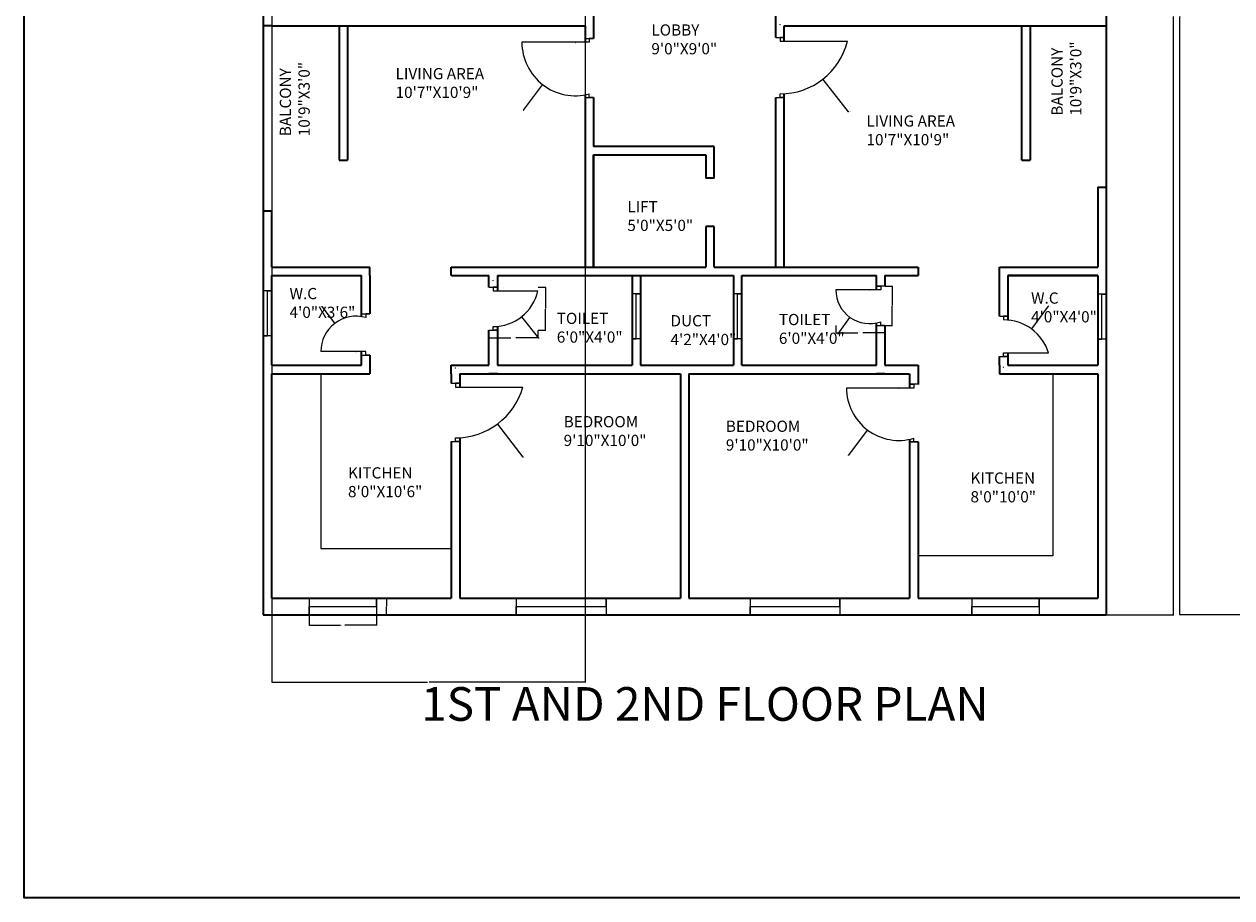
# Model space of a CAD drawing. Units: inches. Extents: x 2043 to 3387, y 1535 to 2797.
# Tile 1 of 7: x 2043 to 2688, y 1535 to 2002. Entities that reach past the tile are written whole.
import ezdxf

# ---------------------------------------------------------------- set-up
doc = ezdxf.new("R2010")
doc.units = ezdxf.units.IN
for name, color, linetype, lineweight in [('A-ANNO-DIMS', 2, 'Continuous', 18), ('A-ANNO-TITL', 7, 'Continuous', 30), ('A-ANNO-TTLB', 7, 'Continuous', 35), ('A-AREA-IDEN', 7, 'Continuous', 18), ('A-DOOR', 3, 'Continuous', 18), ('A-FLOR-FIXT', 9, 'Continuous', 25), ('A-GLAZ', 4, 'Continuous', 18), ('A-WALL', 7, 'Continuous', 35)]:
    doc.layers.add(name, color=color, linetype=linetype, lineweight=lineweight)
doc.styles.get("Standard").update_dxf_attribs({"font": 'arial.ttf'})
doc.dimstyles.get("Standard").update_dxf_attribs({"dimtxt": 0.18, "dimasz": 0.18, "dimexe": 0.18, "dimexo": 0.0625, "dimgap": 0.09, "dimtad": 0, "dimtih": 1, "dimtoh": 1, "dimdec": 4, "dimzin": 0, "dimdsep": 46, "dimtxsty": 'Standard', "dimcen": 0.09, "dimadec": 0, "dimazin": 0, "dimtfac": 1, "dimtdec": 4, "dimtofl": 0, "dimtmove": 0, "dimatfit": 3, "dimfxl": 1, "dimtolj": 1, "dimtzin": 0, "dimarcsym": 0})

# ---------------------------------------------------------------- blocks, each defined once
blk = doc.blocks.new('DOOR-36-ENTRY-SW')
for p, q in [((36, 29.57), (0, 29.57)), ((33.75, 31.57), (38.25, 31.57)), ((38.25, 31.57), (36, 31.57)), ((36, 31.57), (36, 29.57)), ((36, 0), (36, 2)), ((33.75, 0), (38.25, 0)), ((38.25, 0), (36, 0))]:
    blk.add_line(p, q)
blk.add_arc((28.56, 29.57), 28.56, 180, 285.10352)
blk = doc.blocks.new('DOOR-36-ENTRY-SE')
for p, q in [((0, 32.19), (4.5, 32.19)), ((4.5, 32.19), (2.25, 32.19)), ((2.25, 32.19), (2.25, 30.19)), ((2.25, 30.19), (38.25, 30.19)), ((2.25, 0), (2.25, 2)), ((0, 0), (4.5, 0)), ((4.5, 0), (2.25, 0))]:
    blk.add_line(p, q)
blk.add_arc((2.25, 39.08), 37.08, 270, 346.11724)
blk = doc.blocks.new('DOOR-24-WC-SW')
for p, q in [((21.75, 22.19), (26.25, 22.19)), ((26.25, 22.19), (24, 22.19)), ((24, 22.19), (24, 20.19)), ((24, 2), (0, 2)), ((21.75, 0), (26.25, 0)), ((24, 0), (24, 2)), ((26.25, 0), (24, 0))]:
    blk.add_line(p, q)
blk.add_arc((18.89, 2), 18.89, 74.30449, 180)
blk = doc.blocks.new('DOOR-24-BATH-SW')
for p, q in [((0, 23.05), (4.63, 23.05)), ((4.63, 23.05), (2.31, 23.05)), ((2.31, 23.05), (2.31, 21.05)), ((2.31, 21.05), (26.31, 21.05)), ((2.34, 0), (2.34, 2)), ((0.06, 0), (4.63, 0)), ((4.63, 0), (2.34, 0))]:
    blk.add_line(p, q)
blk.add_arc((2.34, 26.6), 24.6, 270, 346.95638)
blk = doc.blocks.new('DOOR-24-BATH-SE')
for p, q in [((26.25, 21.13), (21.75, 21.13)), ((21.75, 21.13), (24, 21.13)), ((24, 21.13), (24, 19.13)), ((24, 19.13), (0, 19.13)), ((24, 0), (24, 2)), ((21.75, 0), (26.25, 0)), ((26.25, 0), (24, 0))]:
    blk.add_line(p, q)
blk.add_arc((18.12, 19.13), 18.12, 180, 288.95077)
blk = doc.blocks.new('DOOR-24-WC-SE')
for p, q in [((0, 21.53), (4.5, 21.53)), ((4.5, 21.53), (2.25, 21.53)), ((2.25, 21.53), (2.25, 19.53)), ((0, 0), (4.5, 0)), ((2.25, 0), (2.25, 2)), ((2.25, 2), (26.25, 2)), ((4.5, 0), (2.25, 0))]:
    blk.add_line(p, q)
blk.add_arc((2.25, -5.66), 25.19, 17.71019, 90)
blk = doc.blocks.new('DOOR-36-BED-SE')
for p, q in [((36, 28.83), (0, 28.83)), ((38.25, 30.83), (33.75, 30.83)), ((33.75, 30.83), (36, 30.83)), ((36, 30.83), (36, 28.83)), ((33.75, 0), (38.25, 0)), ((38.25, 0), (33.75, 0)), ((33.75, 0), (36, 0)), ((36, 0), (36, 2))]:
    blk.add_line(p, q)
blk.add_arc((28, 28.83), 28, 180, 286.60822)
blk = doc.blocks.new('DOOR-36-BED-SW')
for p, q in [((0, 31.2), (4.5, 31.2)), ((4.5, 31.2), (2.25, 31.2)), ((2.25, 31.2), (2.25, 29.2)), ((2.25, 29.2), (38.25, 29.2)), ((0, 0), (4.5, 0)), ((2.25, 0), (2.25, 2)), ((4.5, 0), (2.25, 0))]:
    blk.add_line(p, q)
blk.add_arc((2.25, 39.42), 37.42, 270, 344.14237)
blk = doc.blocks.new('COUNTER-L-SW')
for p, q in [((0, 93.54), (0, 0)), ((0, 0), (69.75, 0))]:
    blk.add_line(p, q)
blk = doc.blocks.new('COUNTER-L-SE')
for p, q in [((72, 97.45), (72, 0)), ((72, 0), (0, 0))]:
    blk.add_line(p, q)
blk = doc.blocks.new('WIN-48-PLAN')
for p, q in [((0, 9), (0, 0)), ((48, 4.5), (48, 9)), ((48, 9), (48, 0)), ((0, 0), (0, 4.5)), ((0, 4.5), (48, 4.5))]:
    blk.add_line(p, q)
blk = doc.blocks.new('VENT-24-PLAN')
for p, q in [((0, 24), (4.5, 24)), ((4.5, 24), (2.25, 24)), ((2.25, 24), (2.25, 0)), ((2.25, 0), (0, 0)), ((0, 0), (4.5, 0))]:
    blk.add_line(p, q)
blk = doc.blocks.new('WIN-36-PLAN')
for p, q in [((0, 9), (0, 0)), ((36, 4.5), (36, 9)), ((36, 9), (36, 0)), ((0, 0), (0, 4.5)), ((0, 4.5), (36, 4.5))]:
    blk.add_line(p, q)
blk = doc.blocks.new('*D39')
at = {"layer": 'A-ANNO-DIMS', "color": 0, "lineweight": -2, "transparency": 16777216}
for p, q in [((2194.81, 1685.81), (2194.81, 1680.3)), ((2230.81, 1685.81), (2230.81, 1680.3)), ((2194.99, 1680.48), (2211.69, 1680.48)), ((2230.63, 1680.48), (2213.93, 1680.48))]:
    blk.add_line(p, q, dxfattribs=at)
at = {"layer": 'A-ANNO-DIMS', "color": 0, "transparency": 16777216}
for points in [[(2194.99, 1680.51), (2194.99, 1680.45), (2194.81, 1680.48)], [(2230.63, 1680.51), (2230.63, 1680.45), (2230.81, 1680.48)]]:
    blk.add_solid(points, dxfattribs=at)
at = {"layer": 'Defpoints', "color": 0, "transparency": 16777216}
for p in [(2194.81, 1685.88), (2230.81, 1685.88), (2230.81, 1680.48)]:
    blk.add_point(p, dxfattribs=at)
at = {"layer": 'A-ANNO-DIMS', "color": 0, "transparency": 16777216, "insert": (2212.81, 1680.48), "char_height": 0.18, "attachment_point": 5}
blk.add_mtext('\\A1;WINDOW 36 TYP.', dxfattribs=at)
blk = doc.blocks.new('*D40')
at = {"layer": 'A-ANNO-DIMS', "color": 0, "lineweight": -2, "transparency": 16777216}
for p, q in [((2230.88, 1694.88), (2236.39, 1694.88)), ((2236.21, 1694.7), (2236.21, 1690.56)), ((2230.88, 1685.88), (2236.39, 1685.88)), ((2236.21, 1686.06), (2236.21, 1690.2))]:
    blk.add_line(p, q, dxfattribs=at)
at = {"layer": 'A-ANNO-DIMS', "color": 0, "transparency": 16777216}
for points in [[(2236.18, 1694.7), (2236.24, 1694.7), (2236.21, 1694.88)], [(2236.18, 1686.06), (2236.24, 1686.06), (2236.21, 1685.88)]]:
    blk.add_solid(points, dxfattribs=at)
at = {"layer": 'Defpoints', "color": 0, "transparency": 16777216}
for p in [(2230.81, 1694.88), (2236.21, 1694.88), (2230.81, 1685.88)]:
    blk.add_point(p, dxfattribs=at)
at = {"layer": 'A-ANNO-DIMS', "color": 0, "transparency": 16777216, "insert": (2236.21, 1690.38), "char_height": 0.18, "attachment_point": 5}
blk.add_mtext('\\A1;9 TYP.', dxfattribs=at)
blk = doc.blocks.new('*D61')
at = {"layer": 'A-ANNO-DIMS', "color": 0, "lineweight": -2, "transparency": 16777216}
for p, q in [((2290.88, 1838.02), (2290.88, 1833.95)), ((2291.06, 1834.13), (2302.73, 1834.13)), ((2317.01, 1834.13), (2305.34, 1834.13)), ((2317.19, 1838.02), (2317.19, 1833.95))]:
    blk.add_line(p, q, dxfattribs=at)
at = {"layer": 'A-ANNO-DIMS', "color": 0, "transparency": 16777216}
for points in [[(2291.06, 1834.16), (2291.06, 1834.1), (2290.88, 1834.13)], [(2317.01, 1834.16), (2317.01, 1834.1), (2317.19, 1834.13)]]:
    blk.add_solid(points, dxfattribs=at)
at = {"layer": 'Defpoints', "color": 0, "transparency": 16777216}
for p in [(2290.88, 1838.08), (2317.19, 1838.08), (2317.19, 1834.13)]:
    blk.add_point(p, dxfattribs=at)
at = {"layer": 'A-ANNO-DIMS', "color": 0, "transparency": 16777216, "insert": (2304.04, 1834.13), "char_height": 0.18, "attachment_point": 5}
blk.add_mtext('\\A1;BATH DOOR 26 TYP.', dxfattribs=at)
blk = doc.blocks.new('*D62')
at = {"layer": 'A-ANNO-DIMS', "color": 0, "lineweight": -2, "transparency": 16777216}
for p, q in [((2317.25, 1861.13), (2321.32, 1861.13)), ((2321.14, 1860.95), (2321.14, 1849.79)), ((2321.14, 1838.26), (2321.14, 1849.42)), ((2317.25, 1838.08), (2321.32, 1838.08))]:
    blk.add_line(p, q, dxfattribs=at)
at = {"layer": 'A-ANNO-DIMS', "color": 0, "transparency": 16777216}
for points in [[(2321.11, 1860.95), (2321.17, 1860.95), (2321.14, 1861.13)], [(2321.11, 1838.26), (2321.17, 1838.26), (2321.14, 1838.08)]]:
    blk.add_solid(points, dxfattribs=at)
at = {"layer": 'Defpoints', "color": 0, "transparency": 16777216}
for p in [(2317.19, 1861.13), (2321.14, 1861.13), (2317.19, 1838.08)]:
    blk.add_point(p, dxfattribs=at)
at = {"layer": 'A-ANNO-DIMS', "color": 0, "transparency": 16777216, "insert": (2321.14, 1849.6), "char_height": 0.18, "attachment_point": 5}
blk.add_mtext('\\A1;23 TYP.', dxfattribs=at)
blk = doc.blocks.new('*D63')
at = {"layer": 'A-ANNO-DIMS', "color": 0, "lineweight": -2, "transparency": 16777216}
for p, q in [((2476.38, 1840.56), (2476.38, 1836.5)), ((2502.63, 1840.56), (2502.63, 1836.5)), ((2476.56, 1836.68), (2488.2, 1836.68)), ((2502.45, 1836.68), (2490.81, 1836.68))]:
    blk.add_line(p, q, dxfattribs=at)
at = {"layer": 'A-ANNO-DIMS', "color": 0, "transparency": 16777216}
for points in [[(2476.56, 1836.71), (2476.56, 1836.65), (2476.38, 1836.68)], [(2502.45, 1836.71), (2502.45, 1836.65), (2502.63, 1836.68)]]:
    blk.add_solid(points, dxfattribs=at)
at = {"layer": 'Defpoints', "color": 0, "transparency": 16777216}
for p in [(2476.38, 1840.62), (2502.63, 1840.62), (2502.63, 1836.68)]:
    blk.add_point(p, dxfattribs=at)
at = {"layer": 'A-ANNO-DIMS', "color": 0, "transparency": 16777216, "insert": (2489.5, 1836.68), "char_height": 0.18, "attachment_point": 5}
blk.add_mtext('\\A1;BATH DOOR 26 TYP.', dxfattribs=at)
blk = doc.blocks.new('*D64')
at = {"layer": 'A-ANNO-DIMS', "color": 0, "lineweight": -2, "transparency": 16777216}
for p, q in [((2502.69, 1861.76), (2506.75, 1861.76)), ((2506.57, 1861.58), (2506.57, 1851.37)), ((2506.57, 1840.8), (2506.57, 1851.01)), ((2502.69, 1840.62), (2506.75, 1840.62))]:
    blk.add_line(p, q, dxfattribs=at)
at = {"layer": 'A-ANNO-DIMS', "color": 0, "transparency": 16777216}
for points in [[(2506.54, 1861.58), (2506.6, 1861.58), (2506.57, 1861.76)], [(2506.54, 1840.8), (2506.6, 1840.8), (2506.57, 1840.62)]]:
    blk.add_solid(points, dxfattribs=at)
at = {"layer": 'Defpoints', "color": 0, "transparency": 16777216}
for p in [(2502.63, 1861.76), (2506.57, 1861.76), (2502.63, 1840.62)]:
    blk.add_point(p, dxfattribs=at)
at = {"layer": 'A-ANNO-DIMS', "color": 0, "transparency": 16777216, "insert": (2506.57, 1851.19), "char_height": 0.18, "attachment_point": 5}
blk.add_mtext('\\A1;21 TYP.', dxfattribs=at)
blk = doc.blocks.new('*D104')
at = {"layer": 'A-ANNO-DIMS', "color": 0, "lineweight": -2, "transparency": 16777216}
for p, q in [((2620.91, 2326.38), (2657.03, 2326.38)), ((2656.85, 2326.2), (2656.85, 2006.31)), ((2656.85, 1686.06), (2656.85, 2005.95)), ((2620.91, 1685.88), (2657.03, 1685.88))]:
    blk.add_line(p, q, dxfattribs=at)
at = {"layer": 'A-ANNO-DIMS', "color": 0, "transparency": 16777216}
for points in [[(2656.82, 2326.2), (2656.88, 2326.2), (2656.85, 2326.38)], [(2656.82, 1686.06), (2656.88, 1686.06), (2656.85, 1685.88)]]:
    blk.add_solid(points, dxfattribs=at)
at = {"layer": 'Defpoints', "color": 0, "transparency": 16777216}
for p in [(2620.85, 2326.38), (2656.85, 2326.38), (2620.85, 1685.88)]:
    blk.add_point(p, dxfattribs=at)
at = {"layer": 'A-ANNO-DIMS', "color": 0, "transparency": 16777216, "insert": (2656.85, 2006.13), "char_height": 0.18, "attachment_point": 5}
blk.add_mtext('\\A1;640.5', dxfattribs=at)
blk = doc.blocks.new('*D106')
at = {"layer": 'A-ANNO-DIMS', "color": 0, "lineweight": -2, "transparency": 16777216}
for p, q in [((2723.65, 2326.38), (2660.13, 2326.38)), ((2660.31, 2326.2), (2660.31, 2006.31)), ((2660.31, 1686.06), (2660.31, 2005.95)), ((2723.65, 1685.88), (2660.13, 1685.88))]:
    blk.add_line(p, q, dxfattribs=at)
at = {"layer": 'A-ANNO-DIMS', "color": 0, "transparency": 16777216}
for points in [[(2660.28, 2326.2), (2660.34, 2326.2), (2660.31, 2326.38)], [(2660.28, 1686.06), (2660.34, 1686.06), (2660.31, 1685.88)]]:
    blk.add_solid(points, dxfattribs=at)
at = {"layer": 'Defpoints', "color": 0, "transparency": 16777216}
for p in [(2660.31, 2326.38), (2723.71, 2326.38), (2723.71, 1685.88)]:
    blk.add_point(p, dxfattribs=at)
at = {"layer": 'A-ANNO-DIMS', "color": 0, "transparency": 16777216, "insert": (2660.31, 2006.13), "char_height": 0.18, "attachment_point": 5}
blk.add_mtext('\\A1;640.5', dxfattribs=at)
blk = doc.blocks.new('*D117')
at = {"layer": 'A-ANNO-DIMS', "color": 0, "lineweight": -2, "transparency": 16777216}
for p, q in [((2174.85, 2134.31), (2174.85, 1649.7)), ((2342.35, 2134.31), (2342.35, 1649.7)), ((2175.03, 1649.88), (2258.21, 1649.88)), ((2342.17, 1649.88), (2258.99, 1649.88))]:
    blk.add_line(p, q, dxfattribs=at)
at = {"layer": 'A-ANNO-DIMS', "color": 0, "transparency": 16777216}
for points in [[(2175.03, 1649.91), (2175.03, 1649.85), (2174.85, 1649.88)], [(2342.17, 1649.91), (2342.17, 1649.85), (2342.35, 1649.88)]]:
    blk.add_solid(points, dxfattribs=at)
at = {"layer": 'Defpoints', "color": 0, "transparency": 16777216}
for p in [(2174.85, 2134.38), (2342.35, 2134.38), (2342.35, 1649.88)]:
    blk.add_point(p, dxfattribs=at)
at = {"layer": 'A-ANNO-DIMS', "color": 0, "transparency": 16777216, "insert": (2258.6, 1649.88), "char_height": 0.18, "attachment_point": 5}
blk.add_mtext('\\A1;167.5', dxfattribs=at)
blk = doc.blocks.new('*D134')
at = {"layer": 'A-ANNO-DIMS', "color": 0, "lineweight": -2, "transparency": 16777216}
for p, q in [((2273.01, 1817.95), (2273.19, 1817.95)), ((2273.1, 1817.86), (2273.1, 1818.04)), ((2309.19, 1770.17), (2295.77, 1787.94)), ((2309.37, 1770.17), (2309.19, 1770.17))]:
    blk.add_line(p, q, dxfattribs=at)
at = {"layer": 'A-ANNO-DIMS', "color": 0, "transparency": 16777216}
blk.add_solid([(2295.79, 1787.96), (2295.74, 1787.93), (2295.66, 1788.09)], dxfattribs=at)
at = {"layer": 'Defpoints', "color": 0, "transparency": 16777216}
for p in [(2273.1, 1817.95), (2295.66, 1788.09)]:
    blk.add_point(p, dxfattribs=at)
at = {"layer": 'A-ANNO-DIMS', "color": 0, "transparency": 16777216, "insert": (2310.12, 1770.17), "char_height": 0.18, "attachment_point": 5}
blk.add_mtext('\\A1;2X R37.424', dxfattribs=at)
blk = doc.blocks.new('*D136')
at = {"layer": 'A-ANNO-DIMS', "color": 0, "lineweight": -2, "transparency": 16777216}
for p, q in [((2446.51, 2001.58), (2446.69, 2001.58)), ((2446.6, 2001.49), (2446.6, 2001.67)), ((2483.18, 1954.87), (2469.57, 1972.24)), ((2483.36, 1954.87), (2483.18, 1954.87))]:
    blk.add_line(p, q, dxfattribs=at)
at = {"layer": 'A-ANNO-DIMS', "color": 0, "transparency": 16777216}
blk.add_solid([(2469.59, 1972.26), (2469.55, 1972.23), (2469.46, 1972.39)], dxfattribs=at)
at = {"layer": 'Defpoints', "color": 0, "transparency": 16777216}
for p in [(2446.6, 2001.58), (2469.46, 1972.39)]:
    blk.add_point(p, dxfattribs=at)
at = {"layer": 'A-ANNO-DIMS', "color": 0, "transparency": 16777216, "insert": (2484.03, 1954.87), "char_height": 0.18, "attachment_point": 5}
blk.add_mtext('\\A1;2X R37.08', dxfattribs=at)
blk = doc.blocks.new('*D138')
at = {"layer": 'A-ANNO-DIMS', "color": 0, "lineweight": -2, "transparency": 16777216}
for p, q in [((2337.07, 1992.07), (2337.25, 1992.07)), ((2337.16, 1991.98), (2337.16, 1992.16)), ((2309.37, 1955.8), (2319.68, 1969.26)), ((2309.19, 1955.8), (2309.37, 1955.8))]:
    blk.add_line(p, q, dxfattribs=at)
at = {"layer": 'A-ANNO-DIMS', "color": 0, "transparency": 16777216}
blk.add_solid([(2319.66, 1969.28), (2319.71, 1969.24), (2319.79, 1969.4)], dxfattribs=at)
at = {"layer": 'Defpoints', "color": 0, "transparency": 16777216}
for p in [(2337.16, 1992.07), (2319.79, 1969.4)]:
    blk.add_point(p, dxfattribs=at)
at = {"layer": 'A-ANNO-DIMS', "color": 0, "transparency": 16777216, "insert": (2308.52, 1955.8), "char_height": 0.18, "attachment_point": 5}
blk.add_mtext('\\A1;2X R28.56', dxfattribs=at)
blk = doc.blocks.new('*D139')
at = {"layer": 'A-ANNO-DIMS', "color": 0, "lineweight": -2, "transparency": 16777216}
for p, q in [((2510.01, 1807.18), (2510.19, 1807.18)), ((2510.1, 1807.09), (2510.1, 1807.27)), ((2483.33, 1771.26), (2493.26, 1784.59)), ((2483.15, 1771.26), (2483.33, 1771.26))]:
    blk.add_line(p, q, dxfattribs=at)
at = {"layer": 'A-ANNO-DIMS', "color": 0, "transparency": 16777216}
blk.add_solid([(2493.24, 1784.61), (2493.28, 1784.57), (2493.37, 1784.73)], dxfattribs=at)
at = {"layer": 'Defpoints', "color": 0, "transparency": 16777216}
for p in [(2510.1, 1807.18), (2493.37, 1784.73)]:
    blk.add_point(p, dxfattribs=at)
at = {"layer": 'A-ANNO-DIMS', "color": 0, "transparency": 16777216, "insert": (2482.65, 1771.26), "char_height": 0.18, "attachment_point": 5}
blk.add_mtext('\\A1;2X R28', dxfattribs=at)
blk = doc.blocks.new('*D142')
at = {"layer": 'A-ANNO-DIMS', "color": 0, "lineweight": -2, "transparency": 16777216}
for p, q in [((2589.88, 1850.98), (2581.07, 1838.92)), ((2590.06, 1850.98), (2589.88, 1850.98)), ((2566.01, 1818.43), (2566.19, 1818.43)), ((2566.1, 1818.34), (2566.1, 1818.52))]:
    blk.add_line(p, q, dxfattribs=at)
at = {"layer": 'A-ANNO-DIMS', "color": 0, "transparency": 16777216}
blk.add_solid([(2581.04, 1838.94), (2581.09, 1838.91), (2580.96, 1838.78)], dxfattribs=at)
at = {"layer": 'Defpoints', "color": 0, "transparency": 16777216}
for p in [(2580.96, 1838.78), (2566.1, 1818.43)]:
    blk.add_point(p, dxfattribs=at)
at = {"layer": 'A-ANNO-DIMS', "color": 0, "transparency": 16777216, "insert": (2590.8, 1850.98), "char_height": 0.18, "attachment_point": 5}
blk.add_mtext('\\A1;2X R25.194', dxfattribs=at)
blk = doc.blocks.new('*D143')
at = {"layer": 'A-ANNO-DIMS', "color": 0, "lineweight": -2, "transparency": 16777216}
for p, q in [((2293.13, 1864.68), (2293.31, 1864.68)), ((2293.22, 1864.59), (2293.22, 1864.77)), ((2317.72, 1833.86), (2308.64, 1845.28)), ((2317.9, 1833.86), (2317.72, 1833.86))]:
    blk.add_line(p, q, dxfattribs=at)
at = {"layer": 'A-ANNO-DIMS', "color": 0, "transparency": 16777216}
blk.add_solid([(2308.67, 1845.3), (2308.62, 1845.26), (2308.53, 1845.42)], dxfattribs=at)
at = {"layer": 'Defpoints', "color": 0, "transparency": 16777216}
for p in [(2293.22, 1864.68), (2308.53, 1845.42)]:
    blk.add_point(p, dxfattribs=at)
at = {"layer": 'A-ANNO-DIMS', "color": 0, "transparency": 16777216, "insert": (2318.64, 1833.86), "char_height": 0.18, "attachment_point": 5}
blk.add_mtext('\\A1;2X R24.603', dxfattribs=at)
blk = doc.blocks.new('*D144')
at = {"layer": 'A-ANNO-DIMS', "color": 0, "lineweight": -2, "transparency": 16777216}
for p, q in [((2201.56, 1850.8), (2201.74, 1850.8)), ((2201.74, 1850.8), (2208.47, 1841.91)), ((2219.9, 1826.71), (2220.08, 1826.71)), ((2219.99, 1826.62), (2219.99, 1826.8))]:
    blk.add_line(p, q, dxfattribs=at)
at = {"layer": 'A-ANNO-DIMS', "color": 0, "transparency": 16777216}
blk.add_solid([(2208.5, 1841.93), (2208.45, 1841.89), (2208.58, 1841.77)], dxfattribs=at)
at = {"layer": 'Defpoints', "color": 0, "transparency": 16777216}
for p in [(2208.58, 1841.77), (2219.99, 1826.71)]:
    blk.add_point(p, dxfattribs=at)
at = {"layer": 'A-ANNO-DIMS', "color": 0, "transparency": 16777216, "insert": (2200.88, 1850.8), "char_height": 0.18, "attachment_point": 5}
blk.add_mtext('\\A1;2X R18.89', dxfattribs=at)
blk = doc.blocks.new('*D146')
at = {"layer": 'A-ANNO-DIMS', "color": 0, "lineweight": -2, "transparency": 16777216}
for p, q in [((2494.4, 1859.76), (2494.58, 1859.76)), ((2494.49, 1859.67), (2494.49, 1859.85)), ((2477.65, 1836.17), (2483.86, 1844.87)), ((2477.47, 1836.17), (2477.65, 1836.17))]:
    blk.add_line(p, q, dxfattribs=at)
at = {"layer": 'A-ANNO-DIMS', "color": 0, "transparency": 16777216}
blk.add_solid([(2483.84, 1844.88), (2483.89, 1844.85), (2483.97, 1845.01)], dxfattribs=at)
at = {"layer": 'Defpoints', "color": 0, "transparency": 16777216}
for p in [(2494.49, 1859.76), (2483.97, 1845.01)]:
    blk.add_point(p, dxfattribs=at)
at = {"layer": 'A-ANNO-DIMS', "color": 0, "transparency": 16777216, "insert": (2476.73, 1836.17), "char_height": 0.18, "attachment_point": 5}
blk.add_mtext('\\A1;2X R18.117', dxfattribs=at)

msp = doc.modelspace()

# ---------------------------------------------------------------- linework, layer by layer
at = {"layer": 'A-ANNO-TTLB'}
msp.add_lwpolyline([(2042.5541, 2796.7818), (3386.9704, 2796.7818), (3386.9704, 1534.5689), (2042.5541, 1534.5689)], close=True, dxfattribs=at)
at = {"layer": 'A-WALL'}
for p, q in [((2170.3496, 2326.3769), (2170.3496, 1734.4589)), ((2620.8496, 2326.3769), (2620.8496, 1685.8769)), ((2346.8496, 2009.0461), (2346.8496, 1994.0737)), ((2444.3496, 1994.6872), (2444.3496, 2009.4195)), ((2174.8496, 2000.8769), (2170.3496, 2000.8769)), ((2174.8496, 2000.8769), (2342.3496, 2000.8769)), ((2210.8496, 2000.8769), (2210.8496, 1929.0247)), ((2215.3496, 2000.8769), (2215.3496, 1929.0247)), ((2342.3496, 2000.8769), (2342.3496, 1992.0737)), ((2448.8496, 2000.8769), (2620.8496, 2000.8769)), ((2448.8496, 1992.6872), (2448.8496, 2000.8769)), ((2575.8496, 1929.0247), (2575.8496, 2000.8769)), ((2580.3496, 2000.8769), (2580.3496, 1929.0247)), ((2342.3496, 1963.9908), (2342.3496, 1871.8769)), ((2346.8496, 1962.5015), (2346.8496, 1936.3769)), ((2444.3496, 1871.8769), (2444.3496, 1962.5015)), ((2448.8496, 1871.8769), (2448.8496, 1964.5698)), ((2411.3496, 1936.3769), (2346.8496, 1936.3769)), ((2346.8496, 1871.8769), (2346.8496, 1931.8769)), ((2346.8496, 1931.8769), (2406.8496, 1931.8769)), ((2346.8496, 1931.8769), (2346.8496, 1871.8769)), ((2406.8496, 1931.8769), (2406.8496, 1919.4326)), ((2411.3496, 1931.8769), (2411.3496, 1936.3769)), ((2411.3496, 1919.4326), (2411.3496, 1931.8769)), ((2210.8496, 1929.0247), (2215.3496, 1929.0247)), ((2575.8496, 1929.0247), (2580.3496, 1929.0247)), ((2411.3496, 1919.4326), (2406.8496, 1919.4326)), ((2616.3496, 1914.5613), (2620.8496, 1914.5613)), ((2616.3496, 1914.5613), (2616.3496, 1871.8769)), ((2174.8496, 1901.8538), (2170.3496, 1901.8538)), ((2174.8496, 1901.8538), (2174.8496, 1871.8769)), ((2411.3496, 1893.5445), (2406.8496, 1893.5445)), ((2406.8496, 1893.5445), (2406.8496, 1871.8769)), ((2411.3496, 1871.8769), (2411.3496, 1893.5445)), ((2174.8496, 1871.8769), (2227.3496, 1871.8769)), ((2174.8496, 1867.3769), (2222.8496, 1867.3769)), ((2174.8496, 1867.3769), (2174.8496, 1819.3769)), ((2222.8496, 1845.3823), (2222.8496, 1867.3769)), ((2227.3496, 1867.3769), (2227.3496, 1871.8769)), ((2227.3496, 1867.3769), (2227.3496, 1846.8958)), ((2270.8496, 1867.3769), (2270.8496, 1871.8769)), ((2270.8496, 1871.8769), (2271.1824, 1871.8769)), ((2271.1824, 1867.3769), (2270.8496, 1867.3769)), ((2271.1824, 1871.8769), (2406.8496, 1871.8769)), ((2271.1824, 1867.3769), (2290.8619, 1867.3769)), ((2290.8789, 1861.1284), (2290.8619, 1867.3769)), ((2295.5051, 1867.3769), (2295.5051, 1859.1284)), ((2295.5051, 1867.3769), (2421.6275, 1867.3769)), ((2367.5051, 1867.3769), (2367.5051, 1819.3769)), ((2372.0051, 1867.3769), (2372.0051, 1819.3769)), ((2411.3496, 1871.8769), (2520.3496, 1871.8769)), ((2421.6275, 1867.3769), (2421.6275, 1819.3769)), ((2426.1275, 1819.3769), (2426.1275, 1867.3769)), ((2426.1275, 1867.3769), (2498.1275, 1867.3769)), ((2498.1275, 1859.7561), (2498.1275, 1867.3769)), ((2502.6275, 1867.3769), (2502.6275, 1861.7561)), ((2502.6275, 1867.3769), (2520.3496, 1867.3769)), ((2520.3496, 1871.8769), (2520.3496, 1867.3769)), ((2563.8496, 1845.6269), (2563.8496, 1871.8769)), ((2563.8496, 1871.8769), (2616.3496, 1871.8769)), ((2616.3496, 1867.3769), (2568.3496, 1867.3769)), ((2568.3496, 1867.3769), (2568.3496, 1843.5263)), ((2568.3496, 1867.3769), (2616.3496, 1867.3769)), ((2616.3496, 1867.3769), (2616.3496, 1819.3769)), ((2295.5051, 1840.1838), (2295.5051, 1819.3769)), ((2498.1275, 1819.3769), (2498.1275, 1842.0077)), ((2502.6275, 1840.6215), (2502.6275, 1819.3769)), ((2290.9928, 1819.3769), (2290.9418, 1838.0778)), ((2222.8496, 1819.3769), (2222.8496, 1826.7103)), ((2227.3496, 1824.7103), (2227.3496, 1814.8769)), ((2563.8496, 1819.3769), (2563.8496, 1824.097)), ((2568.3496, 1826.097), (2568.3496, 1819.3769)), ((2174.8496, 1819.3769), (2222.8496, 1819.3769)), ((2174.8496, 1819.3769), (2222.8496, 1819.3769)), ((2174.8496, 1814.8769), (2227.3496, 1814.8769)), ((2174.8496, 1814.8769), (2174.8496, 1694.8769)), ((2270.8496, 1814.8769), (2270.8496, 1819.3769)), ((2270.8496, 1819.3769), (2271.1824, 1819.3769)), ((2270.8496, 1814.8769), (2270.8496, 1809.7212)), ((2271.1824, 1819.3769), (2290.9928, 1819.3769)), ((2275.3496, 1814.8769), (2393.3496, 1814.8769)), ((2275.3496, 1814.8769), (2275.3496, 1807.7212)), ((2295.5051, 1814.8769), (2291.0051, 1814.8769)), ((2295.5051, 1819.3769), (2367.5051, 1819.3769)), ((2372.0051, 1819.3769), (2421.6275, 1819.3769)), ((2393.3496, 1814.8769), (2393.3496, 1694.8769)), ((2397.8496, 1814.8769), (2397.8496, 1694.8769)), ((2397.8496, 1814.8769), (2515.8496, 1814.8769)), ((2426.1275, 1819.3769), (2498.1275, 1819.3769)), ((2502.6275, 1814.8769), (2498.1275, 1814.8769)), ((2502.6275, 1819.3769), (2520.3496, 1819.3769)), ((2515.8496, 1814.8769), (2515.8496, 1807.1819)), ((2520.3496, 1819.3769), (2520.3496, 1814.8769)), ((2520.3496, 1814.8769), (2520.3496, 1809.1819)), ((2563.8496, 1819.3769), (2563.8496, 1814.8769)), ((2563.8496, 1814.8769), (2616.3496, 1814.8769)), ((2568.3496, 1819.3769), (2616.3496, 1819.3769)), ((2616.3496, 1814.8769), (2616.3496, 1694.8769)), ((2270.8496, 1778.5231), (2270.8496, 1694.8769)), ((2275.3496, 1780.5908), (2275.3496, 1694.8769)), ((2515.8496, 1779.7816), (2515.8496, 1694.8769)), ((2520.3496, 1778.3523), (2520.3496, 1694.8769)), ((2170.3496, 1734.4589), (2170.3496, 1685.8769)), ((2174.8496, 1694.8769), (2270.8496, 1694.8769)), ((2275.3496, 1694.8769), (2393.3496, 1694.8769)), ((2397.8496, 1694.8769), (2515.8496, 1694.8769)), ((2520.3496, 1694.8769), (2616.3496, 1694.8769)), ((2170.3496, 1685.8769), (2620.8496, 1685.8769))]:
    msp.add_line(p, q, dxfattribs=at)

# ---------------------------------------------------------------- block references
at = {"layer": 'A-DOOR'}
for name, p in [('DOOR-36-ENTRY-SE', (2444.35, 1962.502)), ('DOOR-36-ENTRY-SW', (2308.6, 1962.502)), ('DOOR-24-BATH-SW', (2290.879, 1838.078)), ('DOOR-24-BATH-SE', (2476.378, 1840.622)), ('DOOR-24-WC-SW', (2201.1, 1824.71)), ('DOOR-24-WC-SE', (2563.85, 1824.097)), ('DOOR-36-BED-SW', (2270.85, 1778.523)), ('DOOR-36-BED-SE', (2482.1, 1778.352))]:
    msp.add_blockref(name, p, dxfattribs=at)
at = {"layer": 'A-FLOR-FIXT'}
for name, p in [('COUNTER-L-SW', (2201.1, 1721.339)), ('COUNTER-L-SE', (2520.35, 1717.422))]:
    msp.add_blockref(name, p, dxfattribs=at)
at = {"layer": 'A-GLAZ', "rotation": 180}
for p in [(2174.8492, 1859.1776), (2372.0047, 1857.5339), (2426.1271, 1857.5339), (2620.8492, 1857.3829)]:
    msp.add_blockref('VENT-24-PLAN', p, dxfattribs=at)
at = {"layer": 'A-GLAZ'}
for name, p in [('WIN-36-PLAN', (2194.813, 1685.877)), ('WIN-48-PLAN', (2305.5702, 1685.877)), ('WIN-48-PLAN', (2430.5988, 1685.877)), ('WIN-36-PLAN', (2549.0536, 1685.877))]:
    msp.add_blockref(name, p, dxfattribs=at)

# ---------------------------------------------------------------- texts
at = {"layer": 'A-ANNO-TITL', "insert": (2254.7485, 1647.259), "char_height": 18, "attachment_point": 1}
msp.add_mtext_dynamic_manual_height_columns('1ST AND 2ND FLOOR PLAN ', width=337.201444, gutter_width=12.5, heights=[0], dxfattribs=at)
at = {"layer": 'A-AREA-IDEN', "char_height": 6, "attachment_point": 1}
for s, width, insert in [('LOBBY\\P9\'0"X9\'0"', 56.797098, (2377.8159, 2001.6595)), ('LIVING AREA\\P10\'7"X10\'9"', 91.606615, (2241.0992, 1978.323)), ('LIVING AREA\\P10\'7"X10\'9"', 76.864163, (2492.7832, 1953.0112)), ('LIFT\\P5\'0"X5\'0"', 64.152237, (2364.9645, 1907.1871)), ('W.C\\P4\'0"X3\'6"', 70.868554, (2184.4058, 1860.7108)), ('W.C\\P4\'0"X4\'0"', 63.938505, (2580.7582, 1858.3148)), ('TOILET\\P6\'0"X4\'0"', 51.905736, (2327.2488, 1847.4619)), ('DUCT\\P4\'2"X4\'0"', 18.852355, (2388.0295, 1846.1848)), ('TOILET\\P6\'0"X4\'0"', 46.249558, (2445.9583, 1846.8238)), ('BEDROOM\\P9\'10"X10\'0"', 50.484077, (2330.9192, 1792.2017)), ('BEDROOM\\P9\'10"X10\'0"', 100.490059, (2417.6096, 1789.7644)), ('KITCHEN\\P8\'0"X10\'6"', 110.560832, (2215.6592, 1764.8355)), ('KITCHEN\\P8\'0"10\'0"', 109.469008, (2548.3724, 1762.0573))]:
    msp.add_mtext_dynamic_manual_height_columns(s, width=width, gutter_width=12.5, heights=[0], dxfattribs=dict(at, insert=insert))
at = {"layer": 'A-AREA-IDEN', "char_height": 6, "attachment_point": 1, "rotation": 90}
for width, insert in [(84.468691, (2591.6358, 1952.8439)), (67.976492, (2179.1972, 1941.874))]:
    msp.add_mtext_dynamic_manual_height_columns('BALCONY\\P10\'9"X3\'0"', width=width, gutter_width=12.5, heights=[0], dxfattribs=dict(at, insert=insert))

# ---------------------------------------------------------------- dimensions: what is measured, and where the dimension line sits
at = {"layer": 'A-ANNO-DIMS'}
for base, p1, p2, picture, middle in [((2656.8496, 2326.3769), (2620.8496, 1685.8769), (2620.8496, 2326.3769), '*D104', (2656.8496, 2006.1269)), ((2660.3063, 2326.3769), (2723.7086, 1685.8769), (2723.7086, 2326.3769), '*D106', (2660.3063, 2006.1269))]:
    dim = msp.add_linear_dim(base=base, p1=p1, p2=p2, angle=90, dimstyle='Standard', override={"dimdec": 1, "dimlfac": 1, "dimrnd": 0, "dimzin": 0, "dimdsep": 46, "dimlunit": 2}, dxfattribs=at)
    dim.commit()
    dim.dimension.update_dxf_attribs({"geometry": picture, "text_midpoint": middle})
dim = msp.add_linear_dim(base=(2342.3496, 1649.8769), p1=(2174.8496, 2134.3769), p2=(2342.3496, 2134.3769), dimstyle='Standard', override={"dimdec": 1, "dimlfac": 1, "dimrnd": 0, "dimzin": 0, "dimdsep": 46, "dimlunit": 2}, dxfattribs=at)
dim.commit()
dim.dimension.update_dxf_attribs({"geometry": '*D117', "text_midpoint": (2258.5996, 1649.8769)})
for center, mpoint, override, picture, middle in [((2446.5996, 2001.5848), (2469.46, 1972.386), {"dimdec": 2, "dimlfac": 1, "dimrnd": 0, "dimzin": 0, "dimdsep": 46, "dimlunit": 2}, '*D136', (2484.0312, 1954.8667)), ((2337.1583, 1992.0737), (2319.7931, 1969.4011), {"dimdec": 2, "dimlfac": 1, "dimrnd": 0, "dimzin": 0, "dimdsep": 46, "dimlunit": 2}, '*D138', (2308.5192, 1955.7975)), ((2293.2235, 1864.6812), (2308.5323, 1845.4207), {"dimdec": 3, "dimlfac": 1, "dimrnd": 0, "dimzin": 0, "dimdsep": 46, "dimlunit": 2}, '*D143', (2318.6422, 1833.8644)), ((2494.4941, 1859.7561), (2483.967, 1845.012), {"dimdec": 3, "dimlfac": 1, "dimrnd": 0, "dimzin": 0, "dimdsep": 46, "dimlunit": 2}, '*D146', (2476.7261, 1836.1655)), ((2219.9895, 1826.7103), (2208.581, 1841.766), {"dimdec": 2, "dimlfac": 1, "dimrnd": 0, "dimzin": 0, "dimdsep": 46, "dimlunit": 2}, '*D144', (2200.881, 1850.7994)), ((2566.0996, 1818.4329), (2580.9598, 1838.7778), {"dimdec": 3, "dimlfac": 1, "dimrnd": 0, "dimzin": 0, "dimdsep": 46, "dimlunit": 2}, '*D142', (2590.8003, 1850.9847)), ((2273.0996, 1817.9473), (2295.6591, 1788.0869), {"dimdec": 3, "dimlfac": 1, "dimrnd": 0, "dimzin": 0, "dimdsep": 46, "dimlunit": 2}, '*D134', (2310.1191, 1770.1707)), ((2510.0972, 1807.1819), (2493.3669, 1784.7328), {"dimdec": 0, "dimlfac": 1, "dimrnd": 0, "dimzin": 0, "dimdsep": 46, "dimlunit": 2}, '*D139', (2482.6485, 1771.2634))]:
    dim = msp.add_radius_dim(center=center, mpoint=mpoint, text='2X <>', dimstyle='Standard', override=override, dxfattribs=at)
    dim.commit()
    dim.dimension.update_dxf_attribs({"geometry": picture, "text_midpoint": middle, "dimtype": 164})
for base, p1, p2, picture, middle in [((2321.139, 1861.1284), (2317.192, 1838.0778), (2317.192, 1861.1284), '*D62', (2321.139, 1849.6031)), ((2506.565, 1861.7561), (2502.6275, 1840.6215), (2502.6275, 1861.7561), '*D64', (2506.565, 1851.1888)), ((2236.2133, 1694.8769), (2230.8133, 1685.8769), (2230.8133, 1694.8769), '*D40', (2236.2133, 1690.3769))]:
    dim = msp.add_linear_dim(base=base, p1=p1, p2=p2, angle=90, text='<> TYP.', dimstyle='Standard', override={"dimdec": 0, "dimlfac": 1, "dimrnd": 0, "dimzin": 0, "dimdsep": 46, "dimlunit": 2}, dxfattribs=at)
    dim.commit()
    dim.dimension.update_dxf_attribs({"geometry": picture, "text_midpoint": middle})
for base, p1, p2, text, picture, middle in [((2502.6275, 1836.684), (2476.3775, 1840.6215), (2502.6275, 1840.6215), 'BATH DOOR <> TYP.', '*D63', (2489.5025, 1836.684)), ((2317.192, 1834.1308), (2290.8789, 1838.0778), (2317.192, 1838.0778), 'BATH DOOR <> TYP.', '*D61', (2304.0355, 1834.1308)), ((2230.8133, 1680.4769), (2194.8133, 1685.8769), (2230.8133, 1685.8769), 'WINDOW <> TYP.', '*D39', (2212.8133, 1680.4769))]:
    dim = msp.add_linear_dim(base=base, p1=p1, p2=p2, text=text, dimstyle='Standard', override={"dimdec": 0, "dimlfac": 1, "dimrnd": 0, "dimzin": 0, "dimdsep": 46, "dimlunit": 2}, dxfattribs=at)
    dim.commit()
    dim.dimension.update_dxf_attribs({"geometry": picture, "text_midpoint": middle})

doc.saveas('drawing.dxf')
